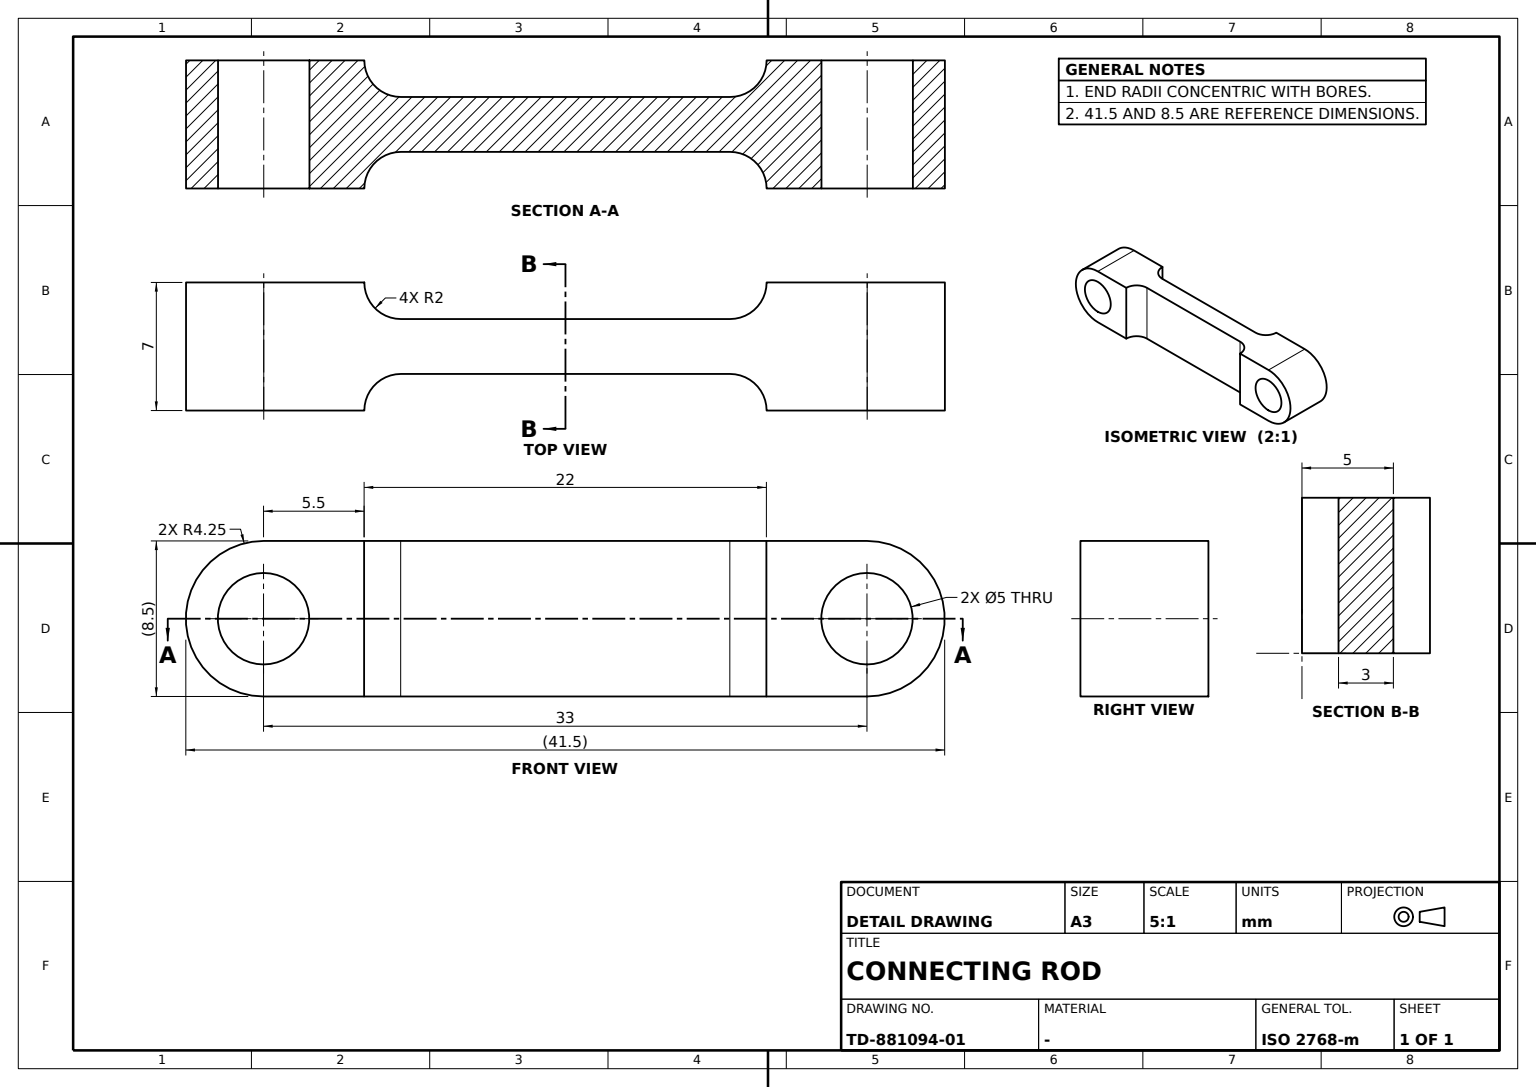
CATIA V5 part; units mm, degrees
sketch "Sketch1" plane through (0, 0, 0) normal (0, 0, 1) x (0, 1, 0)
  point P0 (-11.5, 4.25)
  line L0 (-11.5, 4.25) -> (-16.5, 4.25)
  arc A0 (-16.5, 4.25) -> (-16.5, -4.25) centre (-16.5, 0) ccw
  point P1 (-16.5, 0)
  line L1 (-16.5, -4.25) -> (0, -4.25)
  circle A1 centre (-16.5, 0) radius 2.5
  point P2 (-11.5, 4.25)
  line L2 (-11.5, 4.25) -> (16.5, 4.25)
  arc A2 (16.5, 4.25) -> (16.5, -4.25) centre (16.5, 0) cw
  point P3 (16.5, 0)
  line L3 (16.5, -4.25) -> (0, -4.25)
  circle A3 centre (16.5, 0) radius 2.5
  dimension "radius A0" = 4.25
  dimension "radius A1" = 2.5
  dimension "radius A3" = 2.5
  dimension "distance P1 P3" = 33
  constraint horizontal L0 x-axis
  constraint tangency A0 L0
  constraint tangency L1 A0
  constraint tangency L2 A0
  constraint tangency A2 L1
  constraint tangency A2 L2
  constraint tangency L3 A0
  constraint symmetry L0 L1 x-axis
  constraint symmetry P1 P3 y-axis
  constraint coincidence P2 L0
  constraint coincidence P2 P0
extrude "Pad1" add sketch "Sketch1" along normal mid plane 7
sketch "Sketch2" plane through (4.25, 0, 0) normal (1, 0, 0) x (0, 1, 0)
  line L0 (-11, 7.906) -> (11, 7.906)
  line L1 (11, 7.906) -> (11, 1.5)
  line L2 (11, 1.5) -> (-11, 1.5)
  line L3 (-11, 1.5) -> (-11, 7.906)
  line L4 (0, -3.5) -> (16.5, -3.5) construction
  line L5 (0, 3.5) -> (16.5, 3.5) construction
  dimension "length L0" = 22
  dimension "distance L2 L4" = 5
  dimension "distance L0 L5" = 4.406
  constraint horizontal L0 x-axis
  constraint horizontal L2 x-axis
  constraint vertical L1 y-axis
  constraint vertical L3 y-axis
  constraint symmetry L1 L3 y-axis
extrude "Pocket1" cut sketch "Sketch2" against normal through all
mirror "Mirror1" about plane through (0, 0, 0) normal (0, 0, 1) of "Pocket1"
fillet "Fillet1" radius 2 2 edges at (0, -11, 1.5) (0, 11, 1.5)
fillet "Fillet2" radius 2 2 edges at (0, 11, -1.5) (0, -11, -1.5)
